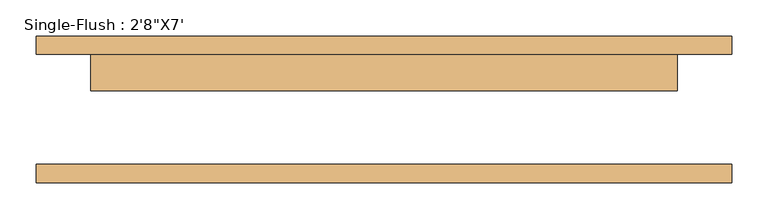
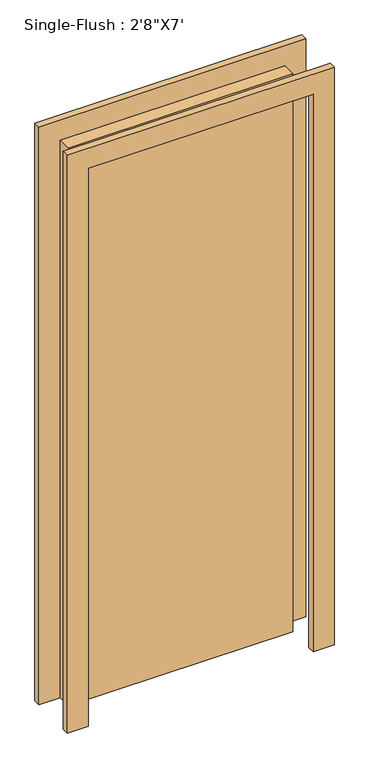
"""IFC4 building model written with IfcOpenShell, lengths in millimetres: door geometry."""

from ifc_helpers import new_model, si_unit, frame, origin, origin_with_axes, place, context, project, spatial, polyline, outline, extrude, source, transform, mapped, element, save


def door_377e7377(model_context):
    return source(origin(), model_context, "Body", "SweptSolid", [
        extrude(outline(polyline([(2209.8, -482.6), (0.0, -482.6), (0.0, -406.4), (2133.6, -406.4), (2133.6, 406.4), (0.0, 406.4), (0.0, 482.6), (2209.8, 482.6), (2209.8, -482.6)])), frame((0.0, 76.2, 0.0), z_axis=(0.0, 1.0, 0.0), x_axis=(0.0, 0.0, 1.0)), (0.0, 0.0, 1.0), 25.4),
        extrude(outline(polyline([(2209.8, 482.6), (2209.8, -482.6), (0.0, -482.6), (0.0, -406.4), (2133.6, -406.4), (2133.6, 406.4), (0.0, 406.4), (0.0, 482.6), (2209.8, 482.6)])), frame((0.0, -101.6, 0.0), z_axis=(0.0, 1.0, 0.0), x_axis=(0.0, 0.0, 1.0)), (0.0, 0.0, 1.0), 25.4),
        extrude(outline(polyline([(406.4, 25.4), (-406.4, 25.4), (-406.4, 76.2), (406.4, 76.2), (406.4, 25.4)])), origin_with_axes(), (0.0, 0.0, 1.0), 2133.6),
    ])


if __name__ == "__main__":
    model = new_model("IFC4")
    model_context = context("Model", 3, world=origin())
    ifc_project = project(units=[si_unit("LENGTHUNIT", "METRE", prefix="MILLI")], contexts=[model_context])
    site = spatial("IfcSite", under=ifc_project)
    building = spatial("IfcBuilding", under=site)
    placement = place(None, origin())
    door_shape = door_377e7377(model_context)
    element("IfcDoor", 1, ObjectType="Single-Flush : 2'8\"X7'", at=placement, inside=building, context=model_context, shape_type="MappedRepresentation", body=[
        mapped(door_shape, transform((0.0, 0.0, 0.0), x_axis=(1.0, 0.0, 0.0), y_axis=(0.0, 1.0, 0.0), z_axis=(0.0, 0.0, 1.0))),
    ])
    save(model, "model.ifc")

# Revit data of these elements
# Type "Single-Flush : 2'8\"X7'"
#   Type Mark = "9"
#   Construction Type Id = "MDOOR"
#   Assembly Code = "C1020"
#   Analytic Construction = "Metal"
#   Thickness = 0' - 2"
#   Heat Transfer Coefficient (U) = 0.651978 BTU/(h·ft²·°F)
#   Height = 7' - 0"
#   Trim Projection Ext = 0' - 1"
#   Trim Projection Int = 0' - 1"
#   Trim Width = 0' - 3"
#   Width = 2' - 8"
#   Define Thermal Properties by = 1
#   Door Material = Door - Panel
#   Frame Material = Door - Frame
#   Visual Light Transmittance = 0
#   Solar Heat Gain Coefficient = 0
#   Function = (empty or 0)
#   Wall Closure = (empty or 0)
# Element 1 (IfcDoor, "Single-Flush : 2'8\"X7'")
#   Materials on its faces: "Door - Frame", "Door - Panel"
# Materials
#   "Door - Panel": class "Wood", colour RGB 210 159 95, transparency 0, Cost = 0
#   "Door - Frame": colour RGB 118 70 51, transparency 0, Cost = 0
